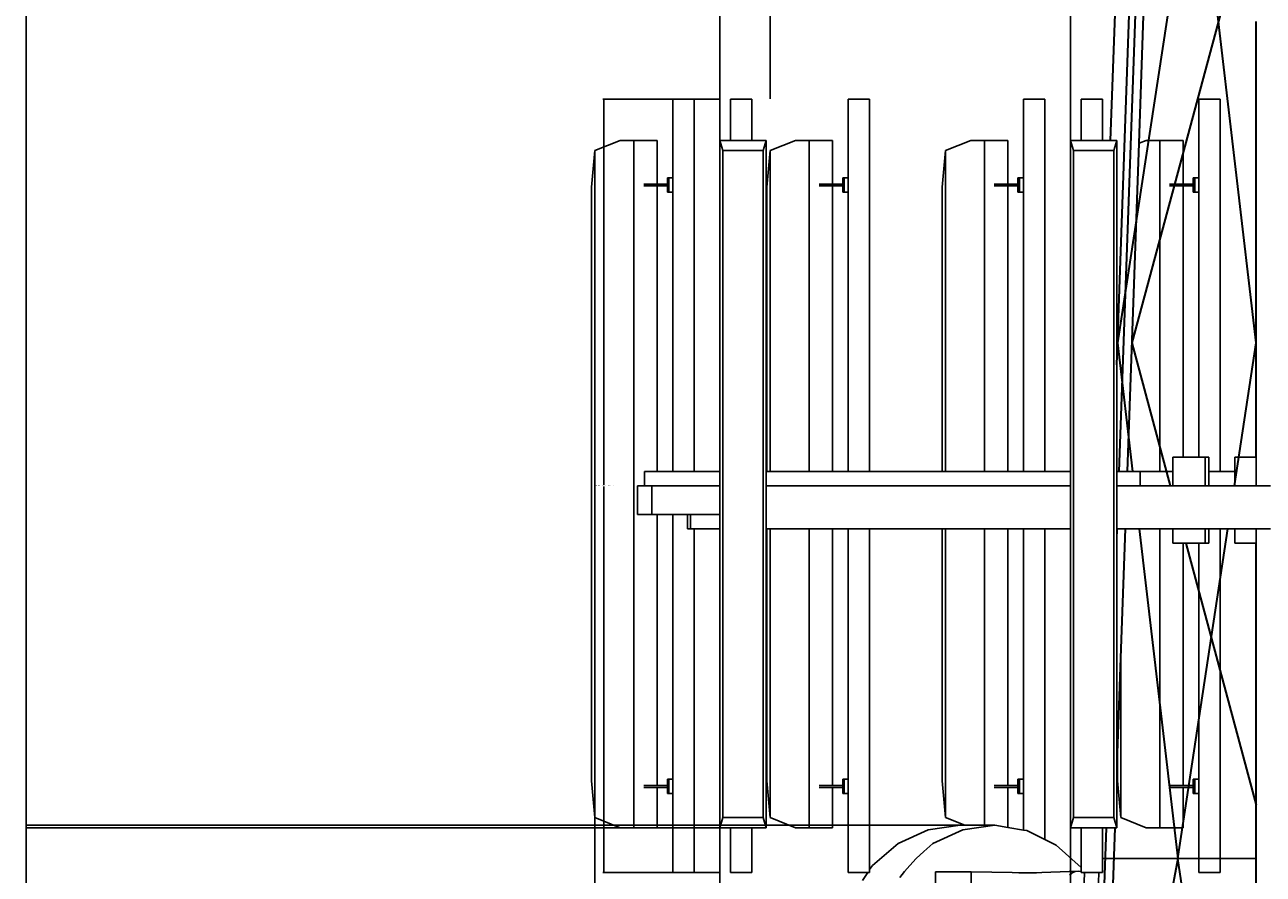
# Model space of a CAD drawing. Units: inches. Extents: x 3780 to 4301, y 1637 to 4224.
# Tile 6 of 8: x 3781 to 4040, y 3682 to 3860. Entities that reach past the tile are written whole.
import ezdxf

# ---------------------------------------------------------------- set-up
doc = ezdxf.new("R2010")
doc.units = ezdxf.units.IN
for name, color, linetype, lineweight in [('A-ANNO-DIMS', 2, 'Continuous', 18), ('E-COMM-ANTN', 4, 'Continuous', 25), ('E-COMM-DISH', 3, 'Continuous', 25), ('S-TOWR', 7, 'Continuous', 35)]:
    doc.layers.add(name, color=color, linetype=linetype, lineweight=lineweight)
doc.styles.get("Standard").update_dxf_attribs({"font": 'arial.ttf'})
doc.dimstyles.get("Standard").update_dxf_attribs({"dimtxt": 0.18, "dimasz": 0.18, "dimexe": 0.18, "dimexo": 0.0625, "dimgap": 0.09, "dimtad": 0, "dimtih": 1, "dimtoh": 1, "dimdec": 4, "dimzin": 0, "dimdsep": 46, "dimtxsty": 'Standard', "dimcen": 0.09, "dimadec": 0, "dimazin": 0, "dimtfac": 1, "dimtdec": 4, "dimtofl": 0, "dimtmove": 0, "dimatfit": 3, "dimfxl": 1, "dimtolj": 1, "dimtzin": 0, "dimarcsym": 0})

# ---------------------------------------------------------------- blocks, each defined once
blk = doc.blocks.new('ANT-PANEL')
for p, q in [((3905.38, 3835.91), (3900.05, 3833.75)), ((3905.38, 3835.91), (3908.22, 3835.91)), ((3908.22, 3691.91), (3908.22, 3835.91)), ((3900.05, 3833.75), (3899.34, 3826.07)), ((3900.05, 3694.07), (3900.05, 3833.75)), ((3899.34, 3701.75), (3899.34, 3826.07)), ((3900.05, 3694.07), (3899.34, 3701.75)), ((3905.38, 3691.91), (3900.05, 3694.07)), ((3905.38, 3691.91), (3908.22, 3691.91))]:
    blk.add_line(p, q)
blk = doc.blocks.new('ANT-PANEL-MOUNT-A')
for p, q in [((3928.47, 3835.91), (3928.47, 3844.56)), ((3928.47, 3844.56), (3932.97, 3844.56)), ((3932.97, 3835.91), (3932.97, 3844.56)), ((3926.23, 3835.91), (3926.9, 3833.75)), ((3926.23, 3835.91), (3928.47, 3835.91)), ((3926.23, 3766.56), (3926.23, 3835.91)), ((3928.47, 3835.91), (3932.97, 3835.91)), ((3932.97, 3835.91), (3935.98, 3835.91)), ((3935.98, 3835.91), (3935.32, 3833.75)), ((3935.98, 3766.56), (3935.98, 3835.91)), ((3926.9, 3694.07), (3926.9, 3833.75)), ((3926.9, 3833.75), (3935.32, 3833.75)), ((3935.32, 3694.07), (3935.32, 3833.75)), ((3936.8, 3833.75), (3936.09, 3826.07)), ((3936.8, 3766.56), (3936.8, 3833.75)), ((3936.09, 3766.56), (3936.09, 3826.07)), ((3926.23, 3763.56), (3926.23, 3766.56)), ((3936.09, 3766.56), (3935.98, 3766.56)), ((3935.98, 3763.56), (3935.98, 3766.56)), ((3936.8, 3766.56), (3936.09, 3766.56)), ((3926.23, 3757.56), (3926.23, 3763.56)), ((3935.98, 3754.56), (3935.98, 3763.56)), ((3926.23, 3754.56), (3926.23, 3757.56)), ((3926.23, 3691.91), (3926.23, 3754.56)), ((3935.98, 3691.91), (3935.98, 3754.56)), ((3935.98, 3754.56), (3936.09, 3754.56)), ((3936.09, 3701.75), (3936.09, 3754.56)), ((3936.09, 3754.56), (3936.8, 3754.56)), ((3936.8, 3694.07), (3936.8, 3754.56)), ((3936.8, 3694.07), (3936.09, 3701.75)), ((3926.23, 3691.91), (3926.9, 3694.07)), ((3926.9, 3694.07), (3935.32, 3694.07)), ((3935.98, 3691.91), (3935.32, 3694.07)), ((3926.23, 3691.91), (3928.47, 3691.91)), ((3928.47, 3682.56), (3928.47, 3691.91)), ((3928.47, 3691.91), (3932.97, 3691.91)), ((3932.97, 3682.56), (3932.97, 3691.91)), ((3932.97, 3691.91), (3935.98, 3691.91)), ((3932.97, 3682.56), (3928.47, 3682.56))]:
    blk.add_line(p, q)
blk = doc.blocks.new('*D7')
at = {"layer": 'A-ANNO-DIMS', "color": 0, "lineweight": -2, "transparency": 16777216}
for p, q in [((3926.17, 3844.56), (3901.75, 3844.56)), ((3901.93, 3844.38), (3901.93, 3763.74)), ((3901.93, 3682.74), (3901.93, 3763.38)), ((3926.17, 3682.56), (3901.75, 3682.56))]:
    blk.add_line(p, q, dxfattribs=at)
at = {"layer": 'A-ANNO-DIMS', "color": 0, "transparency": 16777216}
for points in [[(3901.9, 3844.38), (3901.96, 3844.38), (3901.93, 3844.56)], [(3901.9, 3682.74), (3901.96, 3682.74), (3901.93, 3682.56)]]:
    blk.add_solid(points, dxfattribs=at)
at = {"layer": 'Defpoints', "color": 0, "transparency": 16777216}
for p in [(3901.93, 3844.56), (3926.23, 3844.56), (3926.23, 3682.56)]:
    blk.add_point(p, dxfattribs=at)
at = {"layer": 'A-ANNO-DIMS', "color": 0, "transparency": 16777216, "insert": (3901.93, 3763.56), "char_height": 0.18, "attachment_point": 5}
blk.add_mtext('\\A1;PANEL ANTENNA MOUNT A 162 TYP.', dxfattribs=at)
blk = doc.blocks.new('*D8')
at = {"layer": 'A-ANNO-DIMS', "color": 0, "lineweight": -2, "transparency": 16777216}
for p, q in [((3926.23, 3844.62), (3926.23, 3869.04)), ((3926.41, 3868.86), (3931, 3868.86)), ((3936.62, 3868.86), (3932.03, 3868.86)), ((3936.8, 3844.62), (3936.8, 3869.04))]:
    blk.add_line(p, q, dxfattribs=at)
at = {"layer": 'A-ANNO-DIMS', "color": 0, "transparency": 16777216}
for points in [[(3926.41, 3868.89), (3926.41, 3868.83), (3926.23, 3868.86)], [(3936.62, 3868.89), (3936.62, 3868.83), (3936.8, 3868.86)]]:
    blk.add_solid(points, dxfattribs=at)
at = {"layer": 'Defpoints', "color": 0, "transparency": 16777216}
for p in [(3936.8, 3868.86), (3926.23, 3844.56), (3936.8, 3844.56)]:
    blk.add_point(p, dxfattribs=at)
at = {"layer": 'A-ANNO-DIMS', "color": 0, "transparency": 16777216, "insert": (3931.51, 3868.86), "char_height": 0.18, "attachment_point": 5}
blk.add_mtext('\\A1;11 TYP.', dxfattribs=at)
blk = doc.blocks.new('*D11')
at = {"layer": 'A-ANNO-DIMS', "color": 0, "lineweight": -2, "transparency": 16777216}
for p, q in [((3916.19, 4105.28), (3780.66, 4105.28)), ((3780.84, 4105.1), (3780.84, 2930.44)), ((3780.84, 1755.43), (3780.84, 2930.08)), ((3934.09, 1755.25), (3780.66, 1755.25))]:
    blk.add_line(p, q, dxfattribs=at)
at = {"layer": 'A-ANNO-DIMS', "color": 0, "transparency": 16777216}
for points in [[(3780.81, 4105.1), (3780.87, 4105.1), (3780.84, 4105.28)], [(3780.81, 1755.43), (3780.87, 1755.43), (3780.84, 1755.25)]]:
    blk.add_solid(points, dxfattribs=at)
at = {"layer": 'Defpoints', "color": 0, "transparency": 16777216}
for p in [(3780.84, 4105.28), (3916.25, 4105.28), (3934.15, 1755.25)]:
    blk.add_point(p, dxfattribs=at)
at = {"layer": 'A-ANNO-DIMS', "color": 0, "transparency": 16777216, "insert": (3780.84, 2930.26), "char_height": 0.18, "attachment_point": 5}
blk.add_mtext('\\A1;2350', dxfattribs=at)
blk = doc.blocks.new('*D21')
at = {"layer": 'A-ANNO-DIMS', "color": 0, "lineweight": -2, "transparency": 16777216}
for p, q in [((4010.55, 3901.46), (4300.89, 3901.46)), ((4300.71, 3901.28), (4300.71, 3685.65)), ((4300.71, 3469.64), (4300.71, 3685.28)), ((4044.72, 3469.46), (4300.89, 3469.46))]:
    blk.add_line(p, q, dxfattribs=at)
at = {"layer": 'A-ANNO-DIMS', "color": 0, "transparency": 16777216}
for points in [[(4300.68, 3901.28), (4300.74, 3901.28), (4300.71, 3901.46)], [(4300.68, 3469.64), (4300.74, 3469.64), (4300.71, 3469.46)]]:
    blk.add_solid(points, dxfattribs=at)
at = {"layer": 'Defpoints', "color": 0, "transparency": 16777216}
for p in [(4010.49, 3901.46), (4300.71, 3901.46), (4044.66, 3469.46)]:
    blk.add_point(p, dxfattribs=at)
at = {"layer": 'A-ANNO-DIMS', "color": 0, "transparency": 16777216, "insert": (4300.71, 3685.46), "char_height": 0.18, "attachment_point": 5}
blk.add_mtext('\\A1;432', dxfattribs=at)
blk = doc.blocks.new('*D22')
at = {"layer": 'A-ANNO-DIMS', "color": 0, "lineweight": -2, "transparency": 16777216}
for p, q in [((3900.05, 3694.01), (3900.05, 1636.57)), ((4181.5, 3694.01), (4181.5, 1636.57)), ((3900.23, 1636.75), (4040.31, 1636.75)), ((4181.32, 1636.75), (4041.24, 1636.75))]:
    blk.add_line(p, q, dxfattribs=at)
at = {"layer": 'A-ANNO-DIMS', "color": 0, "transparency": 16777216}
for points in [[(3900.23, 1636.78), (3900.23, 1636.72), (3900.05, 1636.75)], [(4181.32, 1636.78), (4181.32, 1636.72), (4181.5, 1636.75)]]:
    blk.add_solid(points, dxfattribs=at)
at = {"layer": 'Defpoints', "color": 0, "transparency": 16777216}
for p in [(3900.05, 3694.07), (4181.5, 3694.07), (4181.5, 1636.75)]:
    blk.add_point(p, dxfattribs=at)
at = {"layer": 'A-ANNO-DIMS', "color": 0, "transparency": 16777216, "insert": (4040.77, 1636.75), "char_height": 0.18, "attachment_point": 5}
blk.add_mtext('\\A1;281.45', dxfattribs=at)
blk = doc.blocks.new('*D28')
at = {"layer": 'A-ANNO-DIMS', "color": 0, "lineweight": -2, "transparency": 16777216}
for p, q in [((3926.17, 3691.91), (3780.66, 3691.91)), ((3780.84, 3691.73), (3780.84, 3590.48)), ((3780.84, 3488.87), (3780.84, 3590.12)), ((4048.31, 3488.69), (3780.66, 3488.69))]:
    blk.add_line(p, q, dxfattribs=at)
at = {"layer": 'A-ANNO-DIMS', "color": 0, "transparency": 16777216}
for points in [[(3780.81, 3691.73), (3780.87, 3691.73), (3780.84, 3691.91)], [(3780.81, 3488.87), (3780.87, 3488.87), (3780.84, 3488.69)]]:
    blk.add_solid(points, dxfattribs=at)
at = {"layer": 'Defpoints', "color": 0, "transparency": 16777216}
for p in [(3780.84, 3691.91), (3926.23, 3691.91), (4048.37, 3488.69)]:
    blk.add_point(p, dxfattribs=at)
at = {"layer": 'A-ANNO-DIMS', "color": 0, "transparency": 16777216, "insert": (3780.84, 3590.3), "char_height": 0.18, "attachment_point": 5}
blk.add_mtext('\\A1;203.2', dxfattribs=at)
blk = doc.blocks.new('*D29')
at = {"layer": 'A-ANNO-DIMS', "color": 0, "lineweight": -2, "transparency": 16777216}
for p, q in [((3916.19, 4105.28), (3780.66, 4105.28)), ((3780.84, 4105.1), (3780.84, 3898.77)), ((3780.84, 3692.09), (3780.84, 3898.41)), ((3926.17, 3691.91), (3780.66, 3691.91))]:
    blk.add_line(p, q, dxfattribs=at)
at = {"layer": 'A-ANNO-DIMS', "color": 0, "transparency": 16777216}
for points in [[(3780.81, 4105.1), (3780.87, 4105.1), (3780.84, 4105.28)], [(3780.81, 3692.09), (3780.87, 3692.09), (3780.84, 3691.91)]]:
    blk.add_solid(points, dxfattribs=at)
at = {"layer": 'Defpoints', "color": 0, "transparency": 16777216}
for p in [(3780.84, 4105.28), (3916.25, 4105.28), (3926.23, 3691.91)]:
    blk.add_point(p, dxfattribs=at)
at = {"layer": 'A-ANNO-DIMS', "color": 0, "transparency": 16777216, "insert": (3780.84, 3898.59), "char_height": 0.18, "attachment_point": 5}
blk.add_mtext('\\A1;413.4', dxfattribs=at)
blk = doc.blocks.new('*D39')
at = {"layer": 'A-ANNO-DIMS', "color": 0, "lineweight": -2, "transparency": 16777216}
for p, q in [((3926.23, 3835.97), (3926.23, 4223.96)), ((3926.41, 4223.78), (3962.66, 4223.78)), ((3999.55, 4223.78), (3963.31, 4223.78)), ((3999.73, 3835.97), (3999.73, 4223.96))]:
    blk.add_line(p, q, dxfattribs=at)
at = {"layer": 'A-ANNO-DIMS', "color": 0, "transparency": 16777216}
for points in [[(3926.41, 4223.81), (3926.41, 4223.75), (3926.23, 4223.78)], [(3999.55, 4223.81), (3999.55, 4223.75), (3999.73, 4223.78)]]:
    blk.add_solid(points, dxfattribs=at)
at = {"layer": 'Defpoints', "color": 0, "transparency": 16777216}
for p in [(3999.73, 4223.78), (3926.23, 3835.91), (3999.73, 3835.91)]:
    blk.add_point(p, dxfattribs=at)
at = {"layer": 'A-ANNO-DIMS', "color": 0, "transparency": 16777216, "insert": (3962.98, 4223.78), "char_height": 0.18, "attachment_point": 5}
blk.add_mtext('\\A1;73.5', dxfattribs=at)
blk = doc.blocks.new('*D40')
at = {"layer": 'A-ANNO-DIMS', "color": 0, "lineweight": -2, "transparency": 16777216}
for p, q in [((3999.73, 3835.97), (3999.73, 4223.96)), ((3999.91, 4223.78), (4036.16, 4223.78)), ((4073.05, 4223.78), (4036.81, 4223.78)), ((4073.23, 3835.97), (4073.23, 4223.96))]:
    blk.add_line(p, q, dxfattribs=at)
at = {"layer": 'A-ANNO-DIMS', "color": 0, "transparency": 16777216}
for points in [[(3999.91, 4223.81), (3999.91, 4223.75), (3999.73, 4223.78)], [(4073.05, 4223.81), (4073.05, 4223.75), (4073.23, 4223.78)]]:
    blk.add_solid(points, dxfattribs=at)
at = {"layer": 'Defpoints', "color": 0, "transparency": 16777216}
for p in [(4073.23, 4223.78), (3999.73, 3835.91), (4073.23, 3835.91)]:
    blk.add_point(p, dxfattribs=at)
at = {"layer": 'A-ANNO-DIMS', "color": 0, "transparency": 16777216, "insert": (4036.48, 4223.78), "char_height": 0.18, "attachment_point": 5}
blk.add_mtext('\\A1;73.5', dxfattribs=at)
blk = doc.blocks.new('*D43')
at = {"layer": 'A-ANNO-DIMS', "color": 0, "lineweight": -2, "transparency": 16777216}
for p, q in [((3983.82, 3692.42), (3780.66, 3692.42)), ((3780.84, 3692.24), (3780.84, 3662.96)), ((3780.84, 3633.31), (3780.84, 3662.6)), ((3983.19, 3633.13), (3780.66, 3633.13))]:
    blk.add_line(p, q, dxfattribs=at)
at = {"layer": 'A-ANNO-DIMS', "color": 0, "transparency": 16777216}
for points in [[(3780.81, 3692.24), (3780.87, 3692.24), (3780.84, 3692.42)], [(3780.81, 3633.31), (3780.87, 3633.31), (3780.84, 3633.13)]]:
    blk.add_solid(points, dxfattribs=at)
at = {"layer": 'Defpoints', "color": 0, "transparency": 16777216}
for p in [(3983.89, 3692.42), (3780.84, 3633.13), (3983.25, 3633.13)]:
    blk.add_point(p, dxfattribs=at)
at = {"layer": 'A-ANNO-DIMS', "color": 0, "transparency": 16777216, "insert": (3780.84, 3662.78), "char_height": 0.18, "attachment_point": 5}
blk.add_mtext('\\A1;59.29', dxfattribs=at)
blk = doc.blocks.new('*D48')
at = {"layer": 'A-ANNO-DIMS', "color": 0, "lineweight": -2, "transparency": 16777216}
for p, q in [((3926.23, 3245.63), (3926.23, 4223.96)), ((3926.41, 4223.78), (3962.66, 4223.78)), ((3999.55, 4223.78), (3963.31, 4223.78)), ((3999.73, 3245.63), (3999.73, 4223.96))]:
    blk.add_line(p, q, dxfattribs=at)
at = {"layer": 'A-ANNO-DIMS', "color": 0, "transparency": 16777216}
for points in [[(3926.41, 4223.81), (3926.41, 4223.75), (3926.23, 4223.78)], [(3999.55, 4223.81), (3999.55, 4223.75), (3999.73, 4223.78)]]:
    blk.add_solid(points, dxfattribs=at)
at = {"layer": 'Defpoints', "color": 0, "transparency": 16777216}
for p in [(3999.73, 4223.78), (3926.23, 3245.56), (3999.73, 3245.56)]:
    blk.add_point(p, dxfattribs=at)
at = {"layer": 'A-ANNO-DIMS', "color": 0, "transparency": 16777216, "insert": (3962.98, 4223.78), "char_height": 0.18, "attachment_point": 5}
blk.add_mtext('\\A1;73.5', dxfattribs=at)
blk = doc.blocks.new('*D49')
at = {"layer": 'A-ANNO-DIMS', "color": 0, "lineweight": -2, "transparency": 16777216}
for p, q in [((3999.73, 3245.63), (3999.73, 4223.96)), ((3999.91, 4223.78), (4036.16, 4223.78)), ((4073.05, 4223.78), (4036.81, 4223.78)), ((4073.23, 3245.63), (4073.23, 4223.96))]:
    blk.add_line(p, q, dxfattribs=at)
at = {"layer": 'A-ANNO-DIMS', "color": 0, "transparency": 16777216}
for points in [[(3999.91, 4223.81), (3999.91, 4223.75), (3999.73, 4223.78)], [(4073.05, 4223.81), (4073.05, 4223.75), (4073.23, 4223.78)]]:
    blk.add_solid(points, dxfattribs=at)
at = {"layer": 'Defpoints', "color": 0, "transparency": 16777216}
for p in [(4073.23, 4223.78), (3999.73, 3245.56), (4073.23, 3245.56)]:
    blk.add_point(p, dxfattribs=at)
at = {"layer": 'A-ANNO-DIMS', "color": 0, "transparency": 16777216, "insert": (4036.48, 4223.78), "char_height": 0.18, "attachment_point": 5}
blk.add_mtext('\\A1;73.5', dxfattribs=at)

msp = doc.modelspace()

# ---------------------------------------------------------------- linework, layer by layer
at = {"layer": 'E-COMM-ANTN'}
for p, q in [((3916.394, 3828.0582), (3916.394, 3844.5582)), ((3920.894, 3844.5582), (3916.394, 3844.5582)), ((3920.894, 3766.5582), (3920.894, 3844.5582)), ((3953.144, 3828.0582), (3953.144, 3844.5582)), ((3953.144, 3844.5582), (3957.644, 3844.5582)), ((3957.644, 3766.5582), (3957.644, 3844.5582)), ((3989.894, 3828.0582), (3989.894, 3844.5582)), ((3994.394, 3844.5582), (3989.894, 3844.5582)), ((3994.394, 3766.5582), (3994.394, 3844.5582)), ((4001.9676, 3835.9077), (4001.9676, 3844.5582)), ((4006.4676, 3844.5582), (4001.9676, 3844.5582)), ((4006.4676, 3835.9077), (4006.4676, 3844.5582)), ((4026.644, 3828.0582), (4026.644, 3844.5582)), ((4031.144, 3844.5582), (4026.644, 3844.5582)), ((4031.144, 3766.5582), (4031.144, 3844.5582)), ((3913.0928, 3835.9077), (3908.2178, 3835.9077)), ((3913.0928, 3826.7457), (3913.0928, 3835.9077)), ((3942.1336, 3835.9077), (3936.7982, 3833.7477)), ((3942.1336, 3835.9077), (3944.9678, 3835.9077)), ((3944.9678, 3766.5582), (3944.9678, 3835.9077)), ((3949.8428, 3835.9077), (3944.9678, 3835.9077)), ((3949.8428, 3826.7457), (3949.8428, 3835.9077)), ((3978.8836, 3835.9077), (3973.5482, 3833.7477)), ((3978.8836, 3835.9077), (3981.7178, 3835.9077)), ((3981.7178, 3766.5582), (3981.7178, 3835.9077)), ((3986.5928, 3835.9077), (3981.7178, 3835.9077)), ((3986.5928, 3826.7457), (3986.5928, 3835.9077)), ((3999.7315, 3835.9077), (4000.3979, 3833.7477)), ((3999.7315, 3835.9077), (4001.9676, 3835.9077)), ((3999.7315, 3766.5582), (3999.7315, 3835.9077)), ((4001.9676, 3835.9077), (4006.4676, 3835.9077)), ((4006.4676, 3835.9077), (4008.1537, 3835.9077)), ((4008.1537, 3835.9077), (4009.4815, 3835.9077)), ((4009.4815, 3835.9077), (4008.8151, 3833.7477)), ((4009.4815, 3788.8913), (4009.4815, 3835.9077)), ((4015.6336, 3835.9077), (4014.1321, 3835.2998)), ((4015.6336, 3835.9077), (4018.4678, 3835.9077)), ((4018.4678, 3766.5582), (4018.4678, 3835.9077)), ((4023.3428, 3835.9077), (4018.4678, 3835.9077)), ((4023.3428, 3826.7457), (4023.3428, 3835.9077)), ((3973.5482, 3833.7477), (3972.8371, 3826.0653)), ((3973.5482, 3766.5582), (3973.5482, 3833.7477)), ((4000.3979, 3694.0677), (4000.3979, 3833.7477)), ((4000.3979, 3833.7477), (4008.8151, 3833.7477)), ((4008.8151, 3694.0677), (4008.8151, 3833.7477)), ((3915.2457, 3828.0582), (3915.5705, 3828.0582)), ((3915.2457, 3828.0582), (3915.2457, 3826.7457)), ((3915.5705, 3825.0582), (3915.5705, 3828.0582)), ((3915.5705, 3828.0582), (3916.394, 3828.0582)), ((3916.394, 3825.0582), (3916.394, 3828.0582)), ((3951.9957, 3828.0582), (3952.3205, 3828.0582)), ((3951.9957, 3828.0582), (3951.9957, 3826.7457)), ((3952.3205, 3825.0582), (3952.3205, 3828.0582)), ((3952.3205, 3828.0582), (3953.144, 3828.0582)), ((3953.144, 3825.0582), (3953.144, 3828.0582)), ((3988.7457, 3828.0582), (3989.0705, 3828.0582)), ((3988.7457, 3828.0582), (3988.7457, 3826.7457)), ((3989.0705, 3828.0582), (3989.894, 3828.0582)), ((3989.0705, 3825.0582), (3989.0705, 3828.0582)), ((3989.894, 3825.0582), (3989.894, 3828.0582)), ((4025.4957, 3828.0582), (4025.8205, 3828.0582)), ((4025.4957, 3828.0582), (4025.4957, 3826.7457)), ((4025.8205, 3825.0582), (4025.8205, 3828.0582)), ((4025.8205, 3828.0582), (4026.644, 3828.0582)), ((4026.644, 3825.0582), (4026.644, 3828.0582)), ((3910.2873, 3826.7457), (3913.0928, 3826.7457)), ((3910.2873, 3826.3707), (3913.0928, 3826.3707)), ((3915.2457, 3826.7457), (3913.0928, 3826.7457)), ((3913.0928, 3766.5582), (3913.0928, 3826.3707)), ((3913.0928, 3826.3707), (3915.2457, 3826.3707)), ((3915.2457, 3826.7457), (3915.2457, 3826.3707)), ((3915.2457, 3826.3707), (3915.2457, 3825.0582)), ((3915.2457, 3825.0582), (3915.5705, 3825.0582)), ((3915.5705, 3825.0582), (3916.394, 3825.0582)), ((3916.394, 3766.5582), (3916.394, 3825.0582)), ((3949.8428, 3826.7457), (3947.0373, 3826.7457)), ((3947.0373, 3826.3707), (3949.8428, 3826.3707)), ((3951.9957, 3826.7457), (3949.8428, 3826.7457)), ((3949.8428, 3766.5582), (3949.8428, 3826.3707)), ((3949.8428, 3826.3707), (3951.9957, 3826.3707)), ((3951.9957, 3826.7457), (3951.9957, 3826.3707)), ((3951.9957, 3826.3707), (3951.9957, 3825.0582)), ((3951.9957, 3825.0582), (3952.3205, 3825.0582)), ((3952.3205, 3825.0582), (3953.144, 3825.0582)), ((3953.144, 3766.5582), (3953.144, 3825.0582)), ((3972.8371, 3766.5582), (3972.8371, 3826.0653)), ((3983.7873, 3826.7457), (3986.5928, 3826.7457)), ((3983.7873, 3826.3707), (3986.5928, 3826.3707)), ((3988.7457, 3826.7457), (3986.5928, 3826.7457)), ((3986.5928, 3766.5582), (3986.5928, 3826.3707)), ((3986.5928, 3826.3707), (3988.7457, 3826.3707)), ((3988.7457, 3826.7457), (3988.7457, 3826.3707)), ((3988.7457, 3826.3707), (3988.7457, 3825.0582)), ((3988.7457, 3825.0582), (3989.0705, 3825.0582)), ((3989.0705, 3825.0582), (3989.894, 3825.0582)), ((3989.894, 3766.5582), (3989.894, 3825.0582)), ((4020.5373, 3826.7457), (4023.3428, 3826.7457)), ((4020.5373, 3826.3707), (4023.3428, 3826.3707)), ((4025.4957, 3826.7457), (4023.3428, 3826.7457)), ((4023.3428, 3769.5582), (4023.3428, 3826.3707)), ((4023.3428, 3826.3707), (4025.4957, 3826.3707)), ((4025.4957, 3826.7457), (4025.4957, 3826.3707)), ((4025.4957, 3826.3707), (4025.4957, 3825.0582)), ((4025.4957, 3825.0582), (4025.8205, 3825.0582)), ((4025.8205, 3825.0582), (4026.644, 3825.0582)), ((4026.644, 3769.5582), (4026.644, 3825.0582)), ((4009.4815, 3766.5582), (4009.4815, 3788.8913)), ((4021.2379, 3769.5582), (4023.3428, 3769.5582)), ((4021.2379, 3766.5582), (4021.2379, 3769.5582)), ((4023.3428, 3769.5582), (4026.644, 3769.5582)), ((4026.644, 3769.5582), (4027.9879, 3769.5582)), ((4027.9879, 3769.5582), (4028.7541, 3769.5582)), ((4027.9879, 3769.5582), (4027.9879, 3763.5582)), ((4028.7541, 3769.5582), (4028.7541, 3766.5582)), ((4038.6622, 3769.5582), (4034.2176, 3769.5582)), ((4034.2176, 3769.5582), (4034.2176, 3766.5582)), ((4038.6622, 3763.5582), (4038.6622, 3769.5582)), ((3910.4676, 3763.5582), (3910.4676, 3766.5582)), ((3913.0928, 3766.5582), (3910.4676, 3766.5582)), ((3916.394, 3766.5582), (3913.0928, 3766.5582)), ((3920.894, 3766.5582), (3916.394, 3766.5582)), ((3926.2315, 3766.5582), (3920.894, 3766.5582)), ((3944.9678, 3766.5582), (3936.7982, 3766.5582)), ((3949.8428, 3766.5582), (3944.9678, 3766.5582)), ((3953.144, 3766.5582), (3949.8428, 3766.5582)), ((3957.644, 3766.5582), (3953.144, 3766.5582)), ((3972.8371, 3766.5582), (3957.644, 3766.5582)), ((3973.5482, 3766.5582), (3972.8371, 3766.5582)), ((3981.7178, 3766.5582), (3973.5482, 3766.5582)), ((3986.5928, 3766.5582), (3981.7178, 3766.5582)), ((3989.894, 3766.5582), (3986.5928, 3766.5582)), ((3994.394, 3766.5582), (3989.894, 3766.5582)), ((3999.7315, 3766.5582), (3994.394, 3766.5582)), ((3999.7315, 3763.5582), (3999.7315, 3766.5582)), ((4009.9862, 3766.5582), (4009.4815, 3766.5582)), ((4009.4815, 3763.5582), (4009.4815, 3766.5582)), ((4011.6872, 3766.5582), (4009.9862, 3766.5582)), ((4014.3906, 3766.5582), (4011.6872, 3766.5582)), ((4014.3906, 3763.5582), (4014.3906, 3766.5582)), ((4014.3906, 3766.5582), (4018.4678, 3766.5582)), ((4018.4678, 3766.5582), (4021.2379, 3766.5582)), ((4021.2379, 3763.5582), (4021.2379, 3766.5582)), ((4031.144, 3766.5582), (4028.7541, 3766.5582)), ((4028.7541, 3766.5582), (4028.7541, 3763.5582)), ((4034.2176, 3766.5582), (4031.144, 3766.5582)), ((4034.2176, 3766.5582), (4034.2176, 3763.5582)), ((3908.976, 3763.5582), (3910.4676, 3763.5582)), ((3908.976, 3757.5582), (3908.976, 3763.5582)), ((3910.4676, 3763.5582), (3911.9591, 3763.5582)), ((3911.9591, 3763.5582), (3911.9591, 3757.5582)), ((3926.2315, 3763.5582), (3911.9591, 3763.5582)), ((3999.7315, 3763.5582), (3935.9815, 3763.5582)), ((3999.7315, 3754.5582), (3999.7315, 3763.5582)), ((4014.3906, 3763.5582), (4009.4815, 3763.5582)), ((4009.4815, 3754.5582), (4009.4815, 3763.5582)), ((4021.2379, 3763.5582), (4014.3906, 3763.5582)), ((4027.9879, 3763.5582), (4021.2379, 3763.5582)), ((4028.7541, 3763.5582), (4027.9879, 3763.5582)), ((4034.2176, 3763.5582), (4028.7541, 3763.5582)), ((4038.6622, 3763.5582), (4034.2176, 3763.5582)), ((4041.6622, 3763.5582), (4038.6622, 3763.5582)), ((3911.9591, 3757.5582), (3908.976, 3757.5582)), ((3911.9591, 3757.5582), (3913.0928, 3757.5582)), ((3913.0928, 3700.7457), (3913.0928, 3757.5582)), ((3913.0928, 3757.5582), (3916.394, 3757.5582)), ((3916.394, 3702.0582), (3916.394, 3757.5582)), ((3916.394, 3757.5582), (3919.4676, 3757.5582)), ((3919.4676, 3754.5582), (3919.4676, 3757.5582)), ((3919.4676, 3757.5582), (3920.1171, 3757.5582)), ((3920.1171, 3754.5582), (3920.1171, 3757.5582)), ((3920.1171, 3757.5582), (3926.2315, 3757.5582)), ((3920.1171, 3754.5582), (3919.4676, 3754.5582)), ((3920.894, 3754.5582), (3920.1171, 3754.5582)), ((3920.894, 3682.5582), (3920.894, 3754.5582)), ((3926.2315, 3754.5582), (3920.894, 3754.5582)), ((3936.7982, 3754.5582), (3944.9678, 3754.5582)), ((3944.9678, 3691.9077), (3944.9678, 3754.5582)), ((3944.9678, 3754.5582), (3949.8428, 3754.5582)), ((3949.8428, 3700.7457), (3949.8428, 3754.5582)), ((3949.8428, 3754.5582), (3953.144, 3754.5582)), ((3953.144, 3702.0582), (3953.144, 3754.5582)), ((3953.144, 3754.5582), (3957.644, 3754.5582)), ((3957.644, 3683.1335), (3957.644, 3754.5582)), ((3957.644, 3754.5582), (3972.8371, 3754.5582)), ((3972.8371, 3701.7501), (3972.8371, 3754.5582)), ((3972.8371, 3754.5582), (3973.5482, 3754.5582)), ((3973.5482, 3694.0677), (3973.5482, 3754.5582)), ((3973.5482, 3754.5582), (3981.7178, 3754.5582)), ((3981.7178, 3692.421), (3981.7178, 3754.5582)), ((3981.7178, 3754.5582), (3986.5928, 3754.5582)), ((3986.5928, 3700.7457), (3986.5928, 3754.5582)), ((3986.5928, 3754.5582), (3989.894, 3754.5582)), ((3989.894, 3702.0582), (3989.894, 3754.5582)), ((3989.894, 3754.5582), (3994.394, 3754.5582)), ((3994.394, 3689.4408), (3994.394, 3754.5582)), ((3994.394, 3754.5582), (3999.7315, 3754.5582)), ((3999.7315, 3691.9077), (3999.7315, 3754.5582)), ((4009.4815, 3752.3668), (4009.5594, 3754.5582)), ((4009.4815, 3754.5582), (4009.5594, 3754.5582)), ((4009.4815, 3752.3668), (4009.4815, 3754.5582)), ((4009.5594, 3754.5582), (4011.2604, 3754.5582)), ((4011.2604, 3754.5582), (4018.4678, 3754.5582)), ((4018.4678, 3691.9077), (4018.4678, 3754.5582)), ((4018.4678, 3754.5582), (4021.2379, 3754.5582)), ((4021.2379, 3751.5582), (4021.2379, 3754.5582)), ((4021.2379, 3754.5582), (4027.9879, 3754.5582)), ((4027.9879, 3754.5582), (4027.9879, 3751.5582)), ((4027.9879, 3754.5582), (4028.7541, 3754.5582)), ((4028.7541, 3754.5582), (4028.7541, 3751.5582)), ((4028.7541, 3754.5582), (4031.144, 3754.5582)), ((4031.144, 3682.5582), (4031.144, 3754.5582)), ((4034.2176, 3754.5582), (4031.144, 3754.5582)), ((4034.2176, 3754.5582), (4034.2176, 3751.5582)), ((4034.2176, 3754.5582), (4038.6622, 3754.5582)), ((4038.6622, 3751.5582), (4038.6622, 3754.5582)), ((4038.6622, 3754.5582), (4041.6622, 3754.5582)), ((4009.4815, 3704.5416), (4009.4815, 3752.3668)), ((4021.2379, 3751.5582), (4023.3428, 3751.5582)), ((4023.3428, 3700.7457), (4023.3428, 3751.5582)), ((4026.644, 3751.5582), (4023.3428, 3751.5582)), ((4026.644, 3702.0582), (4026.644, 3751.5582)), ((4027.9879, 3751.5582), (4026.644, 3751.5582)), ((4027.9879, 3751.5582), (4028.7541, 3751.5582)), ((4034.2176, 3751.5582), (4038.6622, 3751.5582)), ((4010.2982, 3694.0677), (4010.2982, 3727.5061)), ((4009.4815, 3704.5416), (4009.5871, 3707.5123)), ((4009.5871, 3701.7501), (4009.5871, 3707.5123)), ((4009.4815, 3691.9077), (4009.4815, 3704.5416)), ((3913.0928, 3700.7457), (3910.2873, 3700.7457)), ((3910.2873, 3700.3707), (3913.0928, 3700.3707)), ((3915.2457, 3700.7457), (3913.0928, 3700.7457)), ((3913.0928, 3691.9077), (3913.0928, 3700.3707)), ((3913.0928, 3700.3707), (3915.2457, 3700.3707)), ((3915.2457, 3702.0582), (3915.5705, 3702.0582)), ((3915.2457, 3702.0582), (3915.2457, 3700.7457)), ((3915.2457, 3700.7457), (3915.2457, 3700.3707)), ((3915.2457, 3700.3707), (3915.2457, 3699.0582)), ((3915.5705, 3699.0582), (3915.5705, 3702.0582)), ((3915.5705, 3702.0582), (3916.394, 3702.0582)), ((3916.394, 3699.0582), (3916.394, 3702.0582)), ((3947.0373, 3700.7457), (3949.8428, 3700.7457)), ((3947.0373, 3700.3707), (3949.8428, 3700.3707)), ((3951.9957, 3700.7457), (3949.8428, 3700.7457)), ((3949.8428, 3691.9077), (3949.8428, 3700.3707)), ((3949.8428, 3700.3707), (3951.9957, 3700.3707)), ((3951.9957, 3702.0582), (3952.3205, 3702.0582)), ((3951.9957, 3702.0582), (3951.9957, 3700.7457)), ((3951.9957, 3700.7457), (3951.9957, 3700.3707)), ((3951.9957, 3700.3707), (3951.9957, 3699.0582)), ((3952.3205, 3699.0582), (3952.3205, 3702.0582)), ((3952.3205, 3702.0582), (3953.144, 3702.0582)), ((3953.144, 3699.0582), (3953.144, 3702.0582)), ((3973.5482, 3694.0677), (3972.8371, 3701.7501)), ((3983.7873, 3700.7457), (3986.5928, 3700.7457)), ((3983.7873, 3700.3707), (3986.5928, 3700.3707)), ((3988.7457, 3700.7457), (3986.5928, 3700.7457)), ((3986.5928, 3691.9741), (3986.5928, 3700.3707)), ((3986.5928, 3700.3707), (3988.7457, 3700.3707)), ((3988.7457, 3702.0582), (3989.0705, 3702.0582)), ((3988.7457, 3702.0582), (3988.7457, 3700.7457)), ((3988.7457, 3700.7457), (3988.7457, 3700.3707)), ((3988.7457, 3700.3707), (3988.7457, 3699.0582)), ((3989.0705, 3699.0582), (3989.0705, 3702.0582)), ((3989.0705, 3702.0582), (3989.894, 3702.0582)), ((3989.894, 3699.0582), (3989.894, 3702.0582)), ((4010.2982, 3694.0677), (4009.5871, 3701.7501)), ((4020.5373, 3700.7457), (4023.3428, 3700.7457)), ((4020.5373, 3700.3707), (4023.3428, 3700.3707)), ((4025.4957, 3700.7457), (4023.3428, 3700.7457)), ((4023.3428, 3691.9077), (4023.3428, 3700.3707)), ((4023.3428, 3700.3707), (4025.4957, 3700.3707)), ((4025.4957, 3702.0582), (4025.8205, 3702.0582)), ((4025.4957, 3702.0582), (4025.4957, 3700.7457)), ((4025.4957, 3700.7457), (4025.4957, 3700.3707)), ((4025.4957, 3700.3707), (4025.4957, 3699.0582)), ((4025.8205, 3699.0582), (4025.8205, 3702.0582)), ((4025.8205, 3702.0582), (4026.644, 3702.0582)), ((4026.644, 3699.0582), (4026.644, 3702.0582)), ((3915.2457, 3699.0582), (3915.5705, 3699.0582)), ((3915.5705, 3699.0582), (3916.394, 3699.0582)), ((3916.394, 3682.5582), (3916.394, 3699.0582)), ((3951.9957, 3699.0582), (3952.3205, 3699.0582)), ((3952.3205, 3699.0582), (3953.144, 3699.0582)), ((3953.144, 3682.5582), (3953.144, 3699.0582)), ((3988.7457, 3699.0582), (3989.0705, 3699.0582)), ((3989.0705, 3699.0582), (3989.894, 3699.0582)), ((3989.894, 3691.4292), (3989.894, 3699.0582)), ((4025.4957, 3699.0582), (4025.8205, 3699.0582)), ((4025.8205, 3699.0582), (4026.644, 3699.0582)), ((4026.644, 3682.5582), (4026.644, 3699.0582)), ((3942.1336, 3691.9077), (3936.7982, 3694.0677)), ((3969.9175, 3691.5046), (3976.6256, 3692.421)), ((3977.6156, 3692.421), (3973.5482, 3694.0677)), ((3977.6156, 3692.421), (3976.6256, 3692.421)), ((3977.1778, 3691.5046), (3983.8859, 3692.421)), ((3981.7178, 3692.421), (3977.6156, 3692.421)), ((3983.8859, 3692.421), (3981.7178, 3692.421)), ((3983.8859, 3692.421), (3986.5928, 3691.9741)), ((3986.5928, 3691.9741), (3989.894, 3691.4292)), ((3999.7315, 3691.9077), (4000.3979, 3694.0677)), ((4000.3979, 3694.0677), (4008.8151, 3694.0677)), ((4009.4815, 3691.9077), (4008.8151, 3694.0677)), ((4015.6336, 3691.9077), (4010.2982, 3694.0677)), ((3913.0928, 3691.9077), (3908.2178, 3691.9077)), ((3942.1336, 3691.9077), (3944.9678, 3691.9077)), ((3949.8428, 3691.9077), (3944.9678, 3691.9077)), ((3970.9053, 3688.6306), (3977.1778, 3691.5046)), ((3989.894, 3691.4292), (3990.5724, 3691.3172)), ((3990.5724, 3691.3172), (3994.394, 3689.4408)), ((3999.7315, 3691.9077), (4001.9676, 3691.9077)), ((4001.9676, 3683.5935), (4001.9676, 3691.9077)), ((4001.9676, 3691.9077), (4006.4676, 3691.9077)), ((4006.4676, 3682.5582), (4006.4676, 3691.9077)), ((4006.4676, 3691.9077), (4007.3312, 3691.9077)), ((4007.3312, 3691.9077), (4009.0321, 3691.9077)), ((4009.0321, 3691.9077), (4009.4815, 3691.9077)), ((4015.6336, 3691.9077), (4018.4678, 3691.9077)), ((4023.3428, 3691.9077), (4018.4678, 3691.9077)), ((4006.4676, 3685.4644), (4022.2326, 3685.4644)), ((4038.6622, 3685.4644), (4008.803, 3685.4644)), ((4022.2326, 3685.4644), (4038.6622, 3685.4644)), ((3916.394, 3682.5582), (3920.894, 3682.5582)), ((4026.644, 3682.5582), (4031.144, 3682.5582))]:
    msp.add_line(p, q, dxfattribs=at)
msp.add_lwpolyline([(3958.2356, 3683.9947), (3963.645, 3688.6306), (3969.9175, 3691.5046)], dxfattribs=at)
at = {"layer": 'E-COMM-DISH'}
for p, q in [((3994.394, 3689.4408), (3996.7817, 3688.2684)), ((3996.7817, 3688.2684), (4001.9676, 3683.5935)), ((3953.144, 3682.5582), (3957.2488, 3682.5582)), ((3957.644, 3682.5582), (3957.2488, 3682.5582)), ((3957.644, 3683.1335), (3958.2356, 3683.9947)), ((3957.644, 3682.5582), (3957.644, 3683.1335)), ((3971.4759, 3682.6716), (3971.0873, 3646.2373)), ((3971.4759, 3682.6716), (3978.9667, 3682.6716)), ((3978.9667, 3682.6716), (3978.5781, 3646.2373)), ((3991.8358, 3682.4915), (3978.9667, 3682.6716)), ((3989.135, 3682.4769), (3988.9451, 3682.4761)), ((3989.6141, 3682.4756), (3989.135, 3682.4769)), ((3990.2432, 3682.4719), (3989.6141, 3682.4756)), ((3990.9794, 3682.4659), (3990.2432, 3682.4719)), ((3991.4323, 3682.4615), (3990.9794, 3682.4659)), ((3991.5816, 3682.4826), (3991.4323, 3682.4615)), ((3991.7726, 3682.4581), (3991.4323, 3682.4615)), ((3991.8358, 3682.4915), (3991.5816, 3682.4826)), ((3992.5688, 3682.4491), (3991.7726, 3682.4581)), ((4001.3836, 3682.8261), (3991.8358, 3682.4915)), ((3992.6238, 3682.447), (3992.5688, 3682.4491)), ((3992.6238, 3682.447), (3992.6336, 3682.4482)), ((4000.0735, 3682.4316), (3999.5309, 3681.9506)), ((4000.7054, 3682.7302), (4000.0735, 3682.4316)), ((4001.3836, 3682.8261), (4000.7054, 3682.7302)), ((4001.2675, 3557.9436), (4005.6996, 3682.5582)), ((4001.9676, 3682.7285), (4001.3836, 3682.8261)), ((4001.9676, 3682.7285), (4001.9676, 3683.5935)), ((4001.9676, 3682.5582), (4001.9676, 3682.7285)), ((4001.9676, 3682.5582), (4002.3723, 3682.5582)), ((4002.6939, 3682.398), (4002.3723, 3682.5582)), ((4002.3723, 3682.5582), (4002.6943, 3682.5582)), ((4002.5039, 3677.0562), (4002.6939, 3682.398)), ((4002.6939, 3682.398), (4002.6993, 3682.5505)), ((4002.6943, 3682.5582), (4002.6993, 3682.5505)), ((4002.6943, 3682.5582), (4002.6996, 3682.5582)), ((4002.6993, 3682.5505), (4002.6996, 3682.5582)), ((4002.6996, 3682.5582), (4005.6996, 3682.5582)), ((4005.6996, 3682.5582), (4006.4676, 3682.5582))]:
    msp.add_line(p, q, dxfattribs=at)
for points in [[(3963.9899, 3681.4998), (3964.9416, 3682.7155), (3966.0772, 3684.0217), (3967.4284, 3685.4331), (3969.0271, 3686.9644), (3970.9053, 3688.6306)], [(3956.1368, 3680.8661), (3957.2488, 3682.5582)]]:
    msp.add_lwpolyline(points, dxfattribs=at)
at = {"layer": 'S-TOWR'}
for p, q in [((4038.6622, 3793.4644), (4028.7541, 3878.4687)), ((4034.2176, 3873.7569), (4012.6441, 3793.4644)), ((4008.1537, 3835.9077), (4009.2516, 3866.7769)), ((4009.4815, 3788.8913), (4012.2516, 3866.7769)), ((4020.7969, 3866.7769), (4009.6441, 3793.4644)), ((4009.9862, 3766.5582), (4013.5506, 3866.7769)), ((4014.1321, 3835.2998), (4015.2516, 3866.7769)), ((4038.6622, 3769.5582), (4038.6622, 3860.7769)), ((4011.6872, 3766.5582), (4014.1321, 3835.2998)), ((4009.6441, 3793.4644), (4012.7803, 3766.5582)), ((4012.6441, 3793.4644), (4020.6795, 3763.5582)), ((4034.1127, 3763.5582), (4038.6622, 3793.4644)), ((4010.2982, 3727.5061), (4011.2604, 3754.5582)), ((4014.179, 3754.5582), (4022.2326, 3685.4644)), ((4022.2326, 3685.4644), (4032.7435, 3754.5582)), ((4023.9037, 3751.5582), (4038.6622, 3696.6299)), ((4038.6622, 3588.2865), (4038.6622, 3751.5582)), ((4009.5871, 3707.5123), (4010.2982, 3727.5061)), ((4002.6934, 3561.5086), (4007.3312, 3691.9077)), ((4009.0321, 3691.9077), (4008.2926, 3671.1131)), ((4022.2326, 3685.4644), (4001.9618, 3577.4644)), ((4037.0512, 3588.0544), (4022.2326, 3685.4644))]:
    msp.add_line(p, q, dxfattribs=at)

# ---------------------------------------------------------------- block references
at = {"layer": 'E-COMM-ANTN'}
for name in ['ANT-PANEL-MOUNT-A', 'ANT-PANEL']:
    msp.add_blockref(name, (0, 0), dxfattribs=at)

# ---------------------------------------------------------------- dimensions: what is measured, and where the dimension line sits
at = {"layer": 'A-ANNO-DIMS'}
for base, p1, p2, override, picture, middle in [((3999.7315, 4223.7769), (3926.2315, 3835.9077), (3999.7315, 3835.9077), {"dimdec": 1, "dimlfac": 1, "dimrnd": 0, "dimzin": 0, "dimdsep": 46, "dimlunit": 2}, '*D39', (3962.9815, 4223.7769)), ((3999.7315, 4223.7769), (3926.2315, 3245.5639), (3999.7315, 3245.5639), {"dimdec": 1, "dimlfac": 1, "dimrnd": 0, "dimzin": 0, "dimdsep": 46, "dimlunit": 2}, '*D48', (3962.9815, 4223.7769)), ((4073.2315, 4223.7769), (3999.7315, 3835.9077), (4073.2315, 3835.9077), {"dimdec": 1, "dimlfac": 1, "dimrnd": 0, "dimzin": 0, "dimdsep": 46, "dimlunit": 2}, '*D40', (4036.4815, 4223.7769)), ((4073.2315, 4223.7769), (3999.7315, 3245.5639), (4073.2315, 3245.5639), {"dimdec": 1, "dimlfac": 1, "dimrnd": 0, "dimzin": 0, "dimdsep": 46, "dimlunit": 2}, '*D49', (4036.4815, 4223.7769)), ((4181.498, 1636.7487), (3900.0482, 3694.0677), (4181.498, 3694.0677), {"dimdec": 2, "dimlfac": 1, "dimrnd": 0, "dimzin": 0, "dimdsep": 46, "dimlunit": 2}, '*D22', (4040.7731, 1636.7487))]:
    dim = msp.add_linear_dim(base=base, p1=p1, p2=p2, dimstyle='Standard', override=override, dxfattribs=at)
    dim.commit()
    dim.dimension.update_dxf_attribs({"geometry": picture, "text_midpoint": middle})
for base, p1, p2, override, picture, middle in [((3780.8371, 4105.2769), (3926.2315, 3691.9077), (3916.252, 4105.2769), {"dimdec": 1, "dimlfac": 1, "dimrnd": 0, "dimzin": 0, "dimdsep": 46, "dimlunit": 2}, '*D29', (3780.8371, 3898.5923)), ((3780.8371, 4105.2769), (3934.1525, 1755.2487), (3916.252, 4105.2769), {"dimdec": 0, "dimlfac": 1, "dimrnd": 0, "dimzin": 0, "dimdsep": 46, "dimlunit": 2}, '*D11', (3780.8371, 2930.2628)), ((4300.7091, 3901.4644), (4044.6622, 3469.4644), (4010.4853, 3901.4644), {"dimdec": 0, "dimlfac": 1, "dimrnd": 0, "dimzin": 0, "dimdsep": 46, "dimlunit": 2}, '*D21', (4300.7091, 3685.4644)), ((3780.8371, 3633.1341), (3983.8859, 3692.421), (3983.2536, 3633.1341), {"dimdec": 2, "dimlfac": 1, "dimrnd": 0, "dimzin": 0, "dimdsep": 46, "dimlunit": 2}, '*D43', (3780.8371, 3662.7775)), ((3780.8371, 3691.9077), (4048.3735, 3488.689), (3926.2315, 3691.9077), {"dimdec": 1, "dimlfac": 1, "dimrnd": 0, "dimzin": 0, "dimdsep": 46, "dimlunit": 2}, '*D28', (3780.8371, 3590.2983))]:
    dim = msp.add_linear_dim(base=base, p1=p1, p2=p2, angle=90, dimstyle='Standard', override=override, dxfattribs=at)
    dim.commit()
    dim.dimension.update_dxf_attribs({"geometry": picture, "text_midpoint": middle})
dim = msp.add_linear_dim(base=(3936.7982, 3868.8582), p1=(3926.2315, 3844.5582), p2=(3936.7982, 3844.5582), text='<> TYP.', dimstyle='Standard', override={"dimdec": 0, "dimlfac": 1, "dimrnd": 0, "dimzin": 0, "dimdsep": 46, "dimlunit": 2}, dxfattribs=at)
dim.commit()
dim.dimension.update_dxf_attribs({"geometry": '*D8', "text_midpoint": (3931.5149, 3868.8582)})
dim = msp.add_linear_dim(base=(3901.9315, 3844.5582), p1=(3926.2315, 3682.5582), p2=(3926.2315, 3844.5582), angle=90, text='PANEL ANTENNA MOUNT A <> TYP.', dimstyle='Standard', override={"dimdec": 0, "dimlfac": 1, "dimrnd": 0, "dimzin": 0, "dimdsep": 46, "dimlunit": 2}, dxfattribs=at)
dim.commit()
dim.dimension.update_dxf_attribs({"geometry": '*D7', "text_midpoint": (3901.9315, 3763.5582)})

doc.saveas('drawing.dxf')
